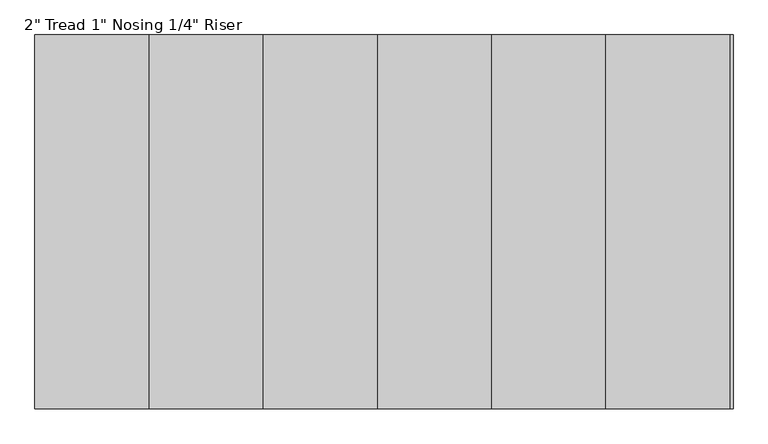
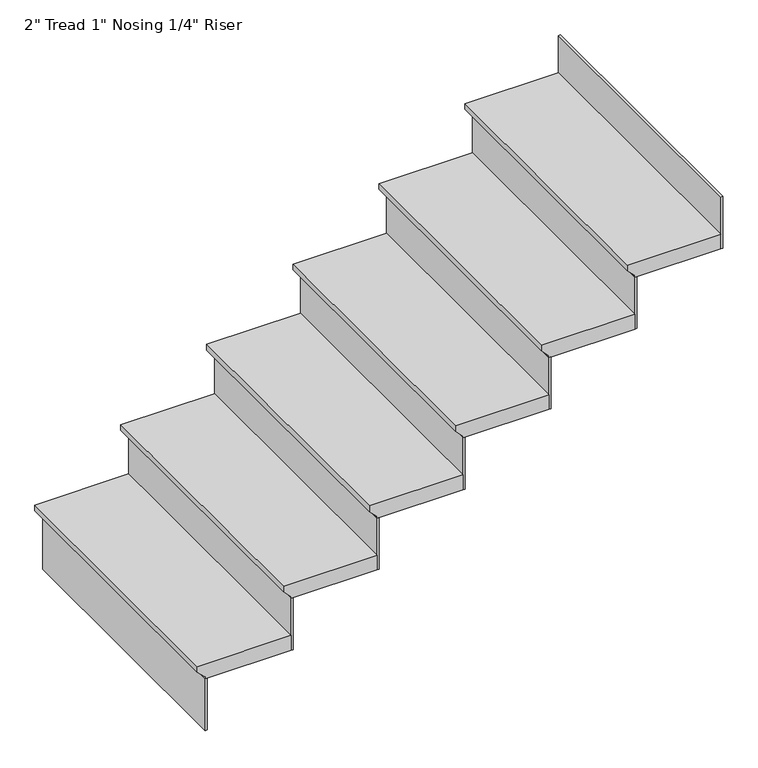
"""IFC4 building model written with IfcOpenShell, lengths in millimetres: stair flight geometry."""

from ifc_helpers import new_model, si_unit, frame, origin, place, context, project, spatial, polyline, outline, extrude, source, transform, mapped, element, save


def stair_flight_b29bf434(model_context):
    return source(origin(), model_context, "Body", "SweptSolid", [
        extrude(outline(polyline([(2743.2, 20511.9136801), (2743.2, 20207.1136801), (2724.15, 20207.1136801), (2698.75, 20232.5136801), (2692.4, 20232.5136801), (2692.4, 20511.9136801), (2743.2, 20511.9136801)])), frame((0.0, 5418.6409313, 0.0), z_axis=(0.0, 1.0, 0.0), x_axis=(0.0, 0.0, 1.0)), (0.0, 0.0, 1.0), 914.4),
        extrude(outline(polyline([(20238.8636801, 5418.6409313), (20232.5136801, 5418.6409313), (20232.5136801, 6333.0409313), (20238.8636801, 6333.0409313), (20238.8636801, 5418.6409313)])), frame((0.0, 0.0, 2514.6), z_axis=(0.0, 0.0, 1.0), x_axis=(1.0, 0.0, 0.0)), (0.0, 0.0, 1.0), 177.8),
        extrude(outline(polyline([(20518.2636801, 5418.6409313), (20511.9136801, 5418.6409313), (20511.9136801, 6333.0409313), (20518.2636801, 6333.0409313), (20518.2636801, 5418.6409313)])), frame((0.0, 0.0, 2692.4), z_axis=(0.0, 0.0, 1.0), x_axis=(1.0, 0.0, 0.0)), (0.0, 0.0, 1.0), 177.8),
        extrude(outline(polyline([(2921.0, 20791.3136801), (2921.0, 20486.5136801), (2901.95, 20486.5136801), (2876.55, 20511.9136801), (2870.2, 20511.9136801), (2870.2, 20791.3136801), (2921.0, 20791.3136801)])), frame((0.0, 5418.6409313, 0.0), z_axis=(0.0, 1.0, 0.0), x_axis=(0.0, 0.0, 1.0)), (0.0, 0.0, 1.0), 914.4),
        extrude(outline(polyline([(20797.6636801, 5418.6409313), (20791.3136801, 5418.6409313), (20791.3136801, 6333.0409313), (20797.6636801, 6333.0409313), (20797.6636801, 5418.6409313)])), frame((0.0, 0.0, 2870.2), z_axis=(0.0, 0.0, 1.0), x_axis=(1.0, 0.0, 0.0)), (0.0, 0.0, 1.0), 177.8),
        extrude(outline(polyline([(3098.8, 21070.7136801), (3098.8, 20765.9136801), (3079.75, 20765.9136801), (3054.35, 20791.3136801), (3048.0, 20791.3136801), (3048.0, 21070.7136801), (3098.8, 21070.7136801)])), frame((0.0, 5418.6409313, 0.0), z_axis=(0.0, 1.0, 0.0), x_axis=(0.0, 0.0, 1.0)), (0.0, 0.0, 1.0), 914.4),
        extrude(outline(polyline([(21077.0636801, 5418.6409313), (21070.7136801, 5418.6409313), (21070.7136801, 6333.0409313), (21077.0636801, 6333.0409313), (21077.0636801, 5418.6409313)])), frame((0.0, 0.0, 3048.0), z_axis=(0.0, 0.0, 1.0), x_axis=(1.0, 0.0, 0.0)), (0.0, 0.0, 1.0), 177.8),
        extrude(outline(polyline([(3276.6, 21350.1136801), (3276.6, 21045.3136801), (3257.55, 21045.3136801), (3232.15, 21070.7136801), (3225.8, 21070.7136801), (3225.8, 21350.1136801), (3276.6, 21350.1136801)])), frame((0.0, 5418.6409313, 0.0), z_axis=(0.0, 1.0, 0.0), x_axis=(0.0, 0.0, 1.0)), (0.0, 0.0, 1.0), 914.4),
        extrude(outline(polyline([(21356.4636801, 5418.6409313), (21350.1136801, 5418.6409313), (21350.1136801, 6333.0409313), (21356.4636801, 6333.0409313), (21356.4636801, 5418.6409313)])), frame((0.0, 0.0, 3225.8), z_axis=(0.0, 0.0, 1.0), x_axis=(1.0, 0.0, 0.0)), (0.0, 0.0, 1.0), 177.8),
        extrude(outline(polyline([(3454.4, 21629.5136801), (3454.4, 21324.7136801), (3435.35, 21324.7136801), (3409.95, 21350.1136801), (3403.6, 21350.1136801), (3403.6, 21629.5136801), (3454.4, 21629.5136801)])), frame((0.0, 5418.6409313, 0.0), z_axis=(0.0, 1.0, 0.0), x_axis=(0.0, 0.0, 1.0)), (0.0, 0.0, 1.0), 914.4),
        extrude(outline(polyline([(21635.8636801, 5418.6409313), (21629.5136801, 5418.6409313), (21629.5136801, 6333.0409313), (21635.8636801, 6333.0409313), (21635.8636801, 5418.6409313)])), frame((0.0, 0.0, 3403.6), z_axis=(0.0, 0.0, 1.0), x_axis=(1.0, 0.0, 0.0)), (0.0, 0.0, 1.0), 177.8),
        extrude(outline(polyline([(21915.2636801, 5418.6409313), (21908.9136801, 5418.6409313), (21908.9136801, 6333.0409313), (21915.2636801, 6333.0409313), (21915.2636801, 5418.6409313)])), frame((0.0, 0.0, 3581.4), z_axis=(0.0, 0.0, 1.0), x_axis=(1.0, 0.0, 0.0)), (0.0, 0.0, 1.0), 177.8),
        extrude(outline(polyline([(3632.2, 21908.9136801), (3632.2, 21604.1136801), (3613.15, 21604.1136801), (3587.75, 21629.5136801), (3581.4, 21629.5136801), (3581.4, 21908.9136801), (3632.2, 21908.9136801)])), frame((0.0, 5418.6409313, 0.0), z_axis=(0.0, 1.0, 0.0), x_axis=(0.0, 0.0, 1.0)), (0.0, 0.0, 1.0), 914.4),
    ])


if __name__ == "__main__":
    model = new_model("IFC4")
    model_context = context("Model", 3, world=origin())
    ifc_project = project(units=[si_unit("LENGTHUNIT", "METRE", prefix="MILLI")], contexts=[model_context])
    site = spatial("IfcSite", under=ifc_project)
    building = spatial("IfcBuilding", under=site)
    placement = place(None, origin())
    stair_flight_shape = stair_flight_b29bf434(model_context)
    element("IfcStairFlight", 1, ObjectType="2\" Tread 1\" Nosing 1/4\" Riser", at=placement, inside=building, context=model_context, shape_type="MappedRepresentation", body=[
        mapped(stair_flight_shape, transform((0.0, 0.0, 0.0), x_axis=(1.0, 0.0, 0.0), y_axis=(0.0, 1.0, 0.0), z_axis=(0.0, 0.0, 1.0))),
    ])
    save(model, "model.ifc")
